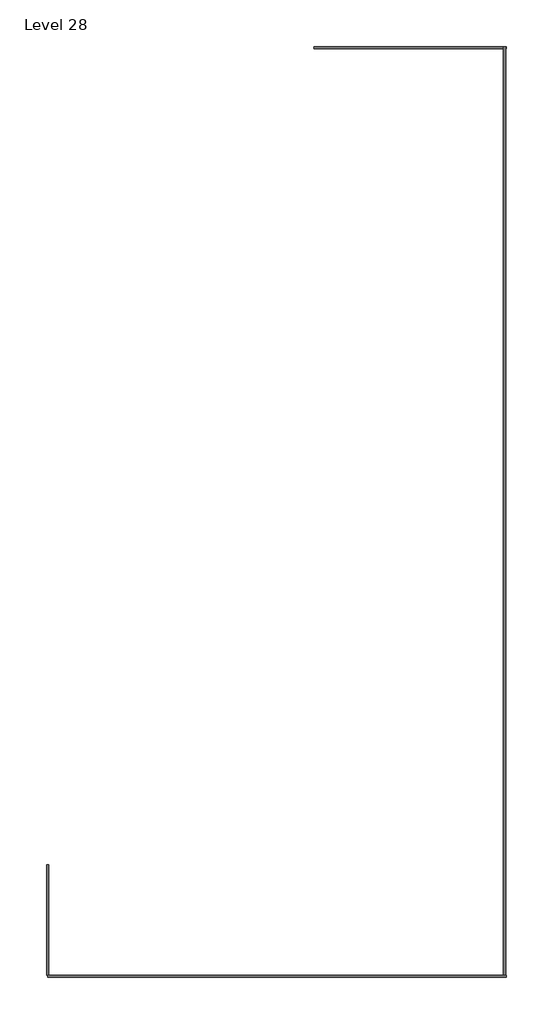
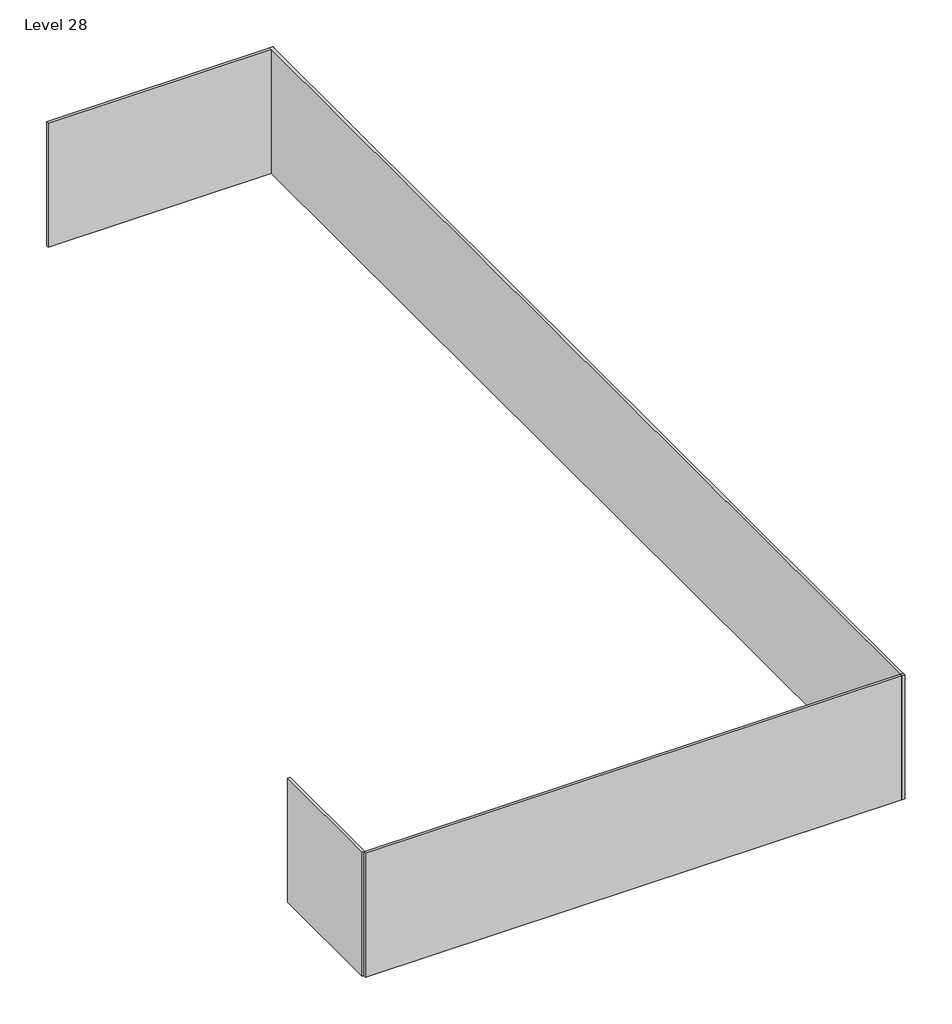
# One storey: 4 plates.
"""IFC4 building model written with IfcOpenShell, lengths in millimetres."""

from ifc_helpers import new_model, si_unit, origin, place, context, project, spatial, transform, mapped, element, save
from components import system_panel_glazed_b1131520, system_panel_glazed_5b5c8ea9, system_panel_glazed_a1bdd1fe, system_panel_glazed_0f25c23b

model = new_model("IFC4")

# Units and contexts
model_context = context("Model", 3, world=origin())
ifc_project = project(units=[si_unit("LENGTHUNIT", "METRE", prefix="MILLI")], contexts=[model_context])

# Site, building, storey
site = spatial("IfcSite", under=ifc_project)
building = spatial("IfcBuilding", under=site)
storey = spatial("IfcBuildingStorey", under=building, Name="Level 28", Elevation=45643.8)

# Plates
placement = place(None, origin())
system_panel_glazed_shape = system_panel_glazed_b1131520(model_context)
element("IfcPlate", 1, ObjectType="System Panel : Glazed", at=placement, inside=storey, context=model_context, shape_type="MappedRepresentation", body=[
    mapped(system_panel_glazed_shape, transform((10041.4464352, -10952.9278294, 45643.8), x_axis=(0.0, -1.0, 0.0), y_axis=(1.0, 0.0, 0.0), z_axis=(0.0, 0.0, 1.0))),
])
system_panel_glazed_2_shape = system_panel_glazed_5b5c8ea9(model_context)
element("IfcPlate", 2, ObjectType="System Panel : Glazed", at=placement, inside=storey, context=model_context, shape_type="MappedRepresentation", body=[
    mapped(system_panel_glazed_2_shape, transform((9038.1464352, -5904.6778294, 45643.8), x_axis=(1.0, 0.0, 0.0), y_axis=(0.0, 1.0, 0.0), z_axis=(0.0, 0.0, 1.0))),
])
system_panel_glazed_3_shape = system_panel_glazed_a1bdd1fe(model_context)
element("IfcPlate", 3, ObjectType="System Panel : Glazed", at=placement, inside=storey, context=model_context, shape_type="MappedRepresentation", body=[
    mapped(system_panel_glazed_3_shape, transform((7581.8430352, -16001.1778294, 45643.8), x_axis=(-1.0, 0.0, 0.0), y_axis=(0.0, -1.0, 0.0), z_axis=(0.0, 0.0, 1.0))),
])
system_panel_glazed_4_shape = system_panel_glazed_0f25c23b(model_context)
element("IfcPlate", 4, ObjectType="System Panel : Glazed", at=placement, inside=storey, context=model_context, shape_type="MappedRepresentation", body=[
    mapped(system_panel_glazed_4_shape, transform((5101.1464352, -15416.9778294, 45643.8), x_axis=(0.0, 1.0, 0.0), y_axis=(-1.0, 0.0, 0.0), z_axis=(0.0, 0.0, 1.0))),
])

save(model, "model.ifc")

# Revit data of these elements
# Type "System Panel : Glazed"
#   Construction Type Id = "GSP4R"
#   Analytic Construction = "1/8 in Pilkington single glazing"
#   Visual Light Transmittance = 0.9
#   Solar Heat Gain Coefficient = 0.86
#   Heat Transfer Coefficient (U) = 1.18115 BTU/(h·ft²·°F)
# Elements 1, 2, 3, 4 (IfcPlate, "System Panel : Glazed")
#   Phase Created = New Construction
#   Materials on its faces: "Glass"
# Materials
#   "Glass": class "Glass", colour RGB 0 128 192, transparency 0.75, Description = "Soda Lime Glass", Cost = 0
